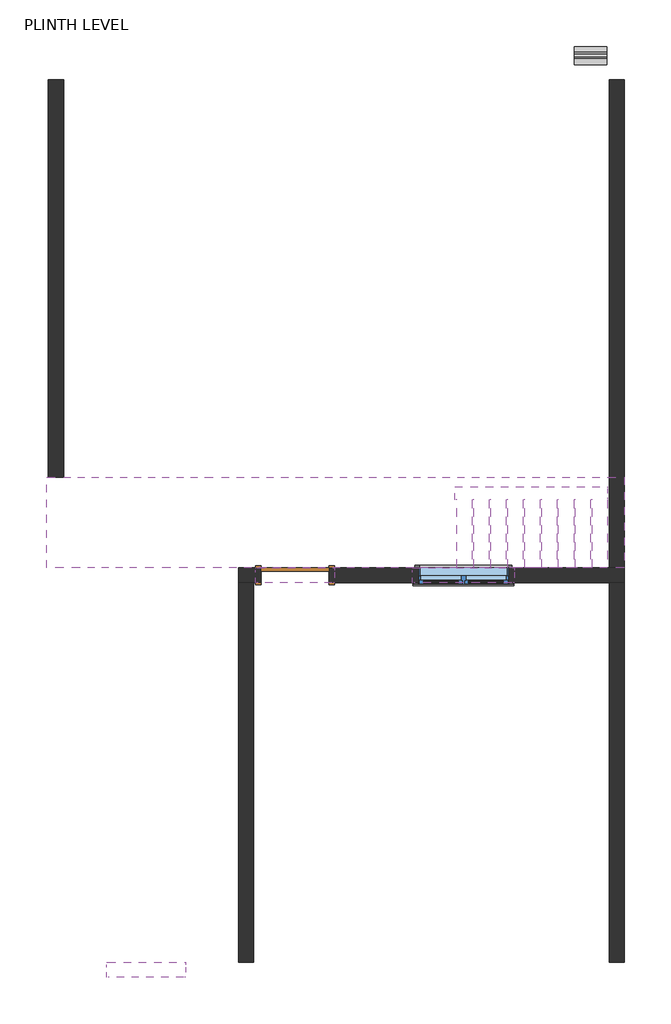
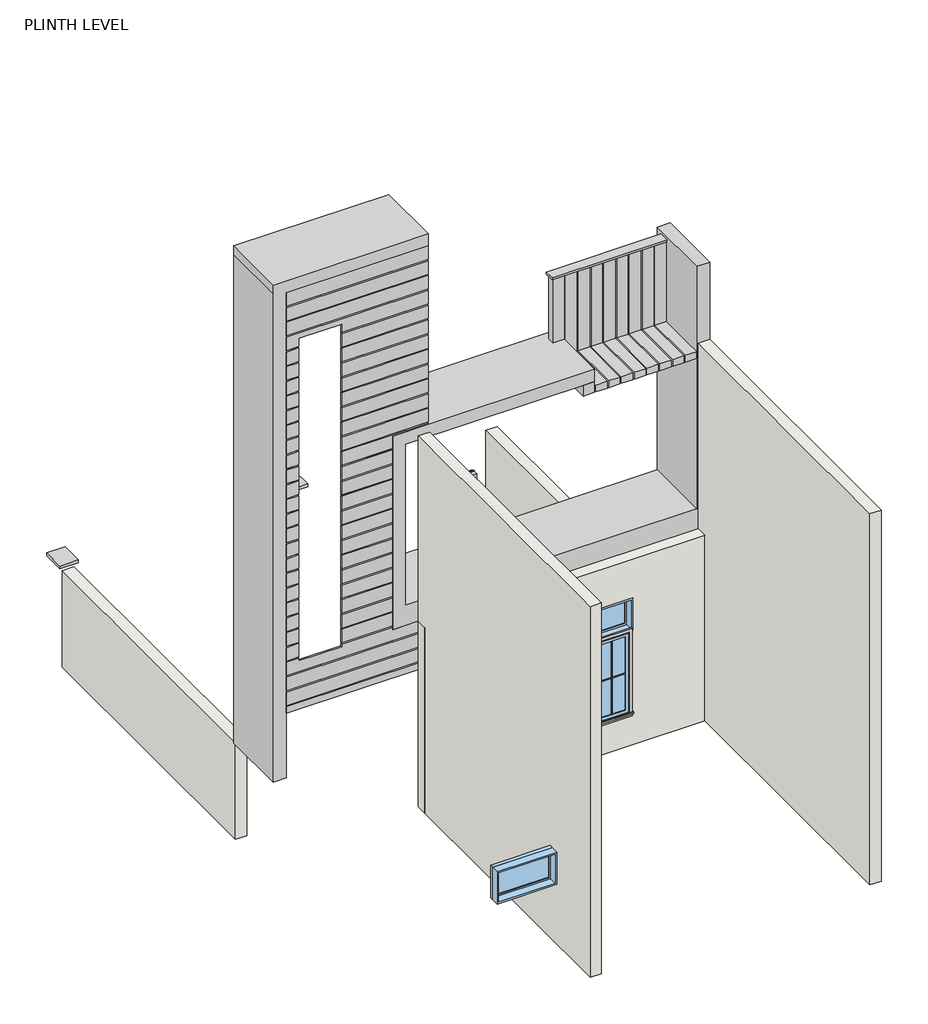
# One storey: 6 proxies, 5 walls, 4 windows, 1 door, 1 light fixture.
"""IFC4 building model written with IfcOpenShell, lengths in millimetres."""

from ifc_helpers import new_model, si_unit, frame, origin, place, context, project, spatial, polyline, outline, extrude, faceted_brep, transform, mapped, element, save
from components import generic_models_4_generic_models_4_1a732ec2, generic_models_6_generic_models_6_807765a8, muntin_pattern_2x2_muntin_pattern_2x2_6dad3731, muntin_pattern_2x2_muntin_pattern_2x2_a30a3345, trim_window_exterior_flat_with_sill_e3be2e48, trim_window_interior_flat_picture_frame_1906adc9, door_54dd4da4, wall_pack_light_exterior_120v_663ef98a, window_e8893895, window_5b0cf282, window_f2c349b1

model = new_model("IFC4")

# Units and contexts
model_context = context("Model", 3, world=origin())
ifc_project = project(units=[si_unit("LENGTHUNIT", "METRE", prefix="MILLI")], contexts=[model_context])

# Site, building, storey
site = spatial("IfcSite", under=ifc_project)
building = spatial("IfcBuilding", under=site)
storey = spatial("IfcBuildingStorey", under=building, Name="PLINTH LEVEL", Elevation=914.4)

# Proxies
placement = place(None, origin())
generic_models_4_generic_models_4_shape = generic_models_4_generic_models_4_1a732ec2(model_context)
element("IfcBuildingElementProxy", 1, Name="Generic Models 4 : Generic Models 4", ObjectType="Generic Models 4 : Generic Models 4", at=placement, inside=storey, context=model_context, shape_type="MappedRepresentation", body=[
    mapped(generic_models_4_generic_models_4_shape, transform((0.0, 0.0, 0.0), x_axis=(1.0, 0.0, 0.0), y_axis=(0.0, 1.0, 0.0), z_axis=(0.0, 0.0, 1.0))),
])
generic_models_6_generic_models_6_shape = generic_models_6_generic_models_6_807765a8(model_context)
element("IfcBuildingElementProxy", 2, Name="Generic Models 6 : Generic Models 6", ObjectType="Generic Models 6 : Generic Models 6", at=placement, inside=storey, context=model_context, shape_type="MappedRepresentation", body=[
    mapped(generic_models_6_generic_models_6_shape, transform((0.0, 0.0, 0.0), x_axis=(1.0, 0.0, 0.0), y_axis=(0.0, 1.0, 0.0), z_axis=(0.0, 0.0, 1.0))),
])
muntin_pattern_2x2_muntin_pattern_2x2_shape = muntin_pattern_2x2_muntin_pattern_2x2_6dad3731(model_context)
element("IfcBuildingElementProxy", 3, Name="Muntin Pattern_2x2 : Muntin Pattern_2x2", ObjectType="Muntin Pattern_2x2 : Muntin Pattern_2x2", at=placement, inside=storey, context=model_context, shape_type="MappedRepresentation", body=[
    mapped(muntin_pattern_2x2_muntin_pattern_2x2_shape, transform((-13781.656205, -12333.7777976, 1619.25), x_axis=(-1.0, 0.0, 0.0), y_axis=(0.0, -1.0, 0.0), z_axis=(0.0, 0.0, 1.0))),
])
muntin_pattern_2x2_muntin_pattern_2x2_2_shape = muntin_pattern_2x2_muntin_pattern_2x2_a30a3345(model_context)
element("IfcBuildingElementProxy", 4, Name="Muntin Pattern_2x2 : Muntin Pattern_2x2", ObjectType="Muntin Pattern_2x2 : Muntin Pattern_2x2", at=placement, inside=storey, context=model_context, shape_type="MappedRepresentation", body=[
    mapped(muntin_pattern_2x2_muntin_pattern_2x2_2_shape, transform((-14388.081205, -12333.7777976, 1619.25), x_axis=(1.0, 0.0, 0.0), y_axis=(0.0, 1.0, 0.0), z_axis=(0.0, 0.0, 1.0))),
])
trim_window_exterior_flat_with_sill_shape = trim_window_exterior_flat_with_sill_e3be2e48(model_context)
element("IfcBuildingElementProxy", 5, Name="Trim-Window-Exterior-Flat : with Sill", ObjectType="Trim-Window-Exterior-Flat : with Sill", at=placement, inside=storey, context=model_context, shape_type="MappedRepresentation", body=[
    mapped(trim_window_exterior_flat_with_sill_shape, transform((-14084.868705, -12343.3027976, 3073.4), x_axis=(-1.0, 0.0, 0.0), y_axis=(0.0, 0.0, -1.0), z_axis=(0.0, -1.0, 0.0))),
])
trim_window_interior_flat_picture_frame_shape = trim_window_interior_flat_picture_frame_1906adc9(model_context)
element("IfcBuildingElementProxy", 6, Name="Trim-Window-Interior-Flat : Picture Frame", ObjectType="Trim-Window-Interior-Flat : Picture Frame", at=placement, inside=storey, context=model_context, shape_type="MappedRepresentation", body=[
    mapped(trim_window_interior_flat_picture_frame_shape, transform((-14084.868705, -12140.1027976, 3073.4), x_axis=(1.0, 0.0, 0.0), y_axis=(0.0, 0.0, -1.0), z_axis=(0.0, 1.0, 0.0))),
])

# Door
door_shape = door_54dd4da4(model_context)
element("IfcDoor", 7, ObjectType="Single-Flush : 36\" x 84\"", at=placement, inside=storey, context=model_context, shape_type="MappedRepresentation", body=[
    mapped(door_shape, transform((-16358.168705, -12241.7027976, 914.4), x_axis=(1.0, 0.0, 0.0), y_axis=(0.0, 1.0, 0.0), z_axis=(0.0, 0.0, 1.0))),
])

# Light fixture
wall_pack_light_exterior_120v_shape = wall_pack_light_exterior_120v_663ef98a(model_context)
element("IfcLightFixture", 8, ObjectType="Wall Pack Light - Exterior : 120V", at=placement, inside=storey, context=model_context, shape_type="MappedRepresentation", body=[
    mapped(wall_pack_light_exterior_120v_shape, transform((-12492.1327615, -5459.9027976, -1390.9222814), x_axis=(1.0, 0.0, 0.0), y_axis=(0.0, 1.0, 0.0), z_axis=(0.0, 0.0, 1.0))),
])

# Walls
element("IfcWall", 9, ObjectType="Generic - 8\"", at=placement, inside=storey, context=model_context, shape_type="SweptSolid", body=[
    extrude(outline(polyline([(-12116.368705, -12140.1027976), (-12116.368705, -5561.5027976), (-11913.168705, -5561.5027976), (-11913.168705, -12140.1027976), (-12116.368705, -12140.1027976)])), frame((0.0, 0.0, 914.4), z_axis=(0.0, 0.0, 1.0), x_axis=(1.0, 0.0, 0.0)), (0.0, 0.0, 1.0), 1371.6),
])
element("IfcWall", 10, ObjectType="Generic - 8\"", at=placement, inside=storey, context=model_context, shape_type="SweptSolid", body=[
    extrude(outline(polyline([(-19482.368705, -5561.5027976), (-19482.368705, -10920.9027976), (-19685.568705, -10920.9027976), (-19685.568705, -5561.5027976), (-19482.368705, -5561.5027976)])), frame((0.0, 0.0, 457.2), z_axis=(0.0, 0.0, 1.0), x_axis=(1.0, 0.0, 0.0)), (0.0, 0.0, 1.0), 1828.8),
])
element("IfcWall", 11, ObjectType="Generic - 8\"", at=placement, inside=storey, context=model_context, shape_type="Brep", body=[
    faceted_brep([(-11913.168705, -17461.4027976, 914.4), (-11913.168705, -12343.3027976, 914.4), (-11913.168705, -12343.3027976, 4419.6), (-11913.168705, -12140.1027976, 4419.6), (-11913.168705, -12140.1027976, 7924.8), (-11913.168705, -17461.4027976, 7924.8), (-12116.368705, -17461.4027976, 914.4), (-12116.368705, -17461.4027976, 7924.8), (-12116.368705, -12343.3027976, 7924.8), (-12116.368705, -12140.1027976, 7924.8), (-12116.368705, -12140.1027976, 4419.6), (-12116.368705, -12343.3027976, 4419.6), (-12116.368705, -12343.3027976, 914.4)], [[[0, 1, 2, 3, 4, 5]], [[6, 7, 8, 9, 10, 11, 12]], [[1, 0, 6, 12]], [[5, 4, 9, 8, 7]], [[0, 5, 7, 6]], [[10, 3, 2, 11]], [[2, 1, 12, 11]], [[4, 3, 10, 9]]]),
])
element("IfcWall", 12, ObjectType="Generic - 8\"", at=placement, inside=storey, context=model_context, shape_type="Brep", body=[
    faceted_brep([(-17120.168705, -12343.3027976, 4419.6), (-17120.168705, -12343.3027976, 914.4), (-17120.168705, -17461.4027976, 914.4), (-17120.168705, -17461.4027976, 7924.8), (-17120.168705, -12140.1027976, 7924.8), (-17120.168705, -12140.1027976, 4419.6), (-16916.968705, -12343.3027976, 914.4), (-16916.968705, -12343.3027976, 4419.6), (-16916.968705, -12140.1027976, 4419.6), (-16916.968705, -12140.1027976, 7924.8), (-16916.968705, -12343.3027976, 7924.8), (-16916.968705, -17461.4027976, 7924.8), (-16916.968705, -17461.4027976, 914.4)], [[[0, 1, 2, 3, 4, 5]], [[6, 7, 8, 9, 10, 11, 12]], [[2, 1, 6, 12]], [[4, 3, 11, 10, 9]], [[5, 8, 7, 0]], [[0, 7, 6, 1]], [[5, 4, 9, 8]], [[3, 2, 12, 11]]]),
])
element("IfcWall", 13, ObjectType="Generic - 8\" 2", at=placement, inside=storey, context=model_context, shape_type="Brep", body=[
    faceted_brep([(-17120.168705, -12140.1027976, 4419.6), (-16916.968705, -12140.1027976, 4419.6), (-16815.368705, -12140.1027976, 4419.6), (-15900.968705, -12140.1027976, 4419.6), (-12116.368705, -12140.1027976, 4419.6), (-11913.168705, -12140.1027976, 4419.6), (-11913.168705, -12140.1027976, 2286.0), (-11913.168705, -12140.1027976, 914.4), (-12116.368705, -12140.1027976, 914.4), (-15900.968705, -12140.1027976, 914.4), (-15900.968705, -12140.1027976, 3048.0), (-16815.368705, -12140.1027976, 3048.0), (-16815.368705, -12140.1027976, 914.4), (-17120.168705, -12140.1027976, 914.4), (-17120.168705, -12140.1027976, 3505.2), (-15824.768705, -12140.1027976, 3067.05), (-15824.768705, -12140.1027976, 3676.65), (-16891.568705, -12140.1027976, 3676.65), (-16891.568705, -12140.1027976, 3067.05), (-13399.068705, -12140.1027976, 3073.4), (-13399.068705, -12140.1027976, 3683.0), (-14770.668705, -12140.1027976, 3683.0), (-14770.668705, -12140.1027976, 3073.4), (-14694.468705, -12140.1027976, 3073.4), (-14694.468705, -12140.1027976, 1549.4), (-13475.268705, -12140.1027976, 1549.4), (-13475.268705, -12140.1027976, 3073.4), (-11913.168705, -12343.3027976, 4419.6), (-12116.368705, -12343.3027976, 4419.6), (-15900.968705, -12343.3027976, 4419.6), (-16815.368705, -12343.3027976, 4419.6), (-16916.968705, -12343.3027976, 4419.6), (-17120.168705, -12343.3027976, 4419.6), (-17120.168705, -12343.3027976, 3505.2), (-17120.168705, -12343.3027976, 914.4), (-16916.968705, -12343.3027976, 914.4), (-16815.368705, -12343.3027976, 914.4), (-16815.368705, -12343.3027976, 3048.0), (-15900.968705, -12343.3027976, 3048.0), (-15900.968705, -12343.3027976, 914.4), (-12116.368705, -12343.3027976, 914.4), (-11913.168705, -12343.3027976, 914.4), (-15824.768705, -12343.3027976, 3676.65), (-15824.768705, -12343.3027976, 3067.05), (-16891.568705, -12343.3027976, 3067.05), (-16891.568705, -12343.3027976, 3676.65), (-13399.068705, -12343.3027976, 3683.0), (-13399.068705, -12343.3027976, 3073.4), (-13475.268705, -12343.3027976, 3073.4), (-13475.268705, -12343.3027976, 1549.4), (-14694.468705, -12343.3027976, 1549.4), (-14694.468705, -12343.3027976, 3073.4), (-14770.668705, -12343.3027976, 3073.4), (-14770.668705, -12343.3027976, 3683.0)], [[[0, 1, 2, 3, 4, 5, 6, 7, 8, 9, 10, 11, 12, 13, 14], [15, 16, 17, 18], [19, 20, 21, 22, 23, 24, 25, 26]], [[27, 28, 29, 30, 31, 32, 33, 34, 35, 36, 37, 38, 39, 40, 41], [42, 43, 44, 45], [46, 47, 48, 49, 50, 51, 52, 53]], [[39, 9, 8, 7, 41, 40]], [[12, 36, 35, 34, 13]], [[5, 4, 3, 2, 1, 0, 32, 31, 30, 29, 28, 27]], [[10, 9, 39, 38]], [[11, 10, 38, 37]], [[12, 11, 37, 36]], [[42, 16, 15, 43]], [[43, 15, 18, 44]], [[44, 18, 17, 45]], [[16, 42, 45, 17]], [[47, 46, 20, 19]], [[47, 19, 26, 48]], [[22, 52, 51, 23]], [[53, 52, 22, 21]], [[46, 53, 21, 20]], [[25, 49, 48, 26]], [[49, 25, 24, 50]], [[50, 24, 23, 51]], [[5, 27, 41, 7, 6]], [[13, 34, 33, 32, 0, 14]]]),
])

# Windows
window_shape = window_e8893895(model_context)
element("IfcWindow", 14, ObjectType="Fixed : 42\" x 24\"", at=placement, inside=storey, context=model_context, shape_type="MappedRepresentation", body=[
    mapped(window_shape, transform((-18326.668705, -17563.0027976, 914.4), x_axis=(1.0, 0.0, 0.0), y_axis=(0.0, 1.0, 0.0), z_axis=(0.0, 0.0, 1.0))),
])
element("IfcWindow", 15, ObjectType="Fixed : 42\" x 24\"", at=placement, inside=storey, context=model_context, shape_type="MappedRepresentation", body=[
    mapped(window_shape, transform((-16320.068705, -12241.7027976, 933.45), x_axis=(1.0, 0.0, 0.0), y_axis=(0.0, 1.0, 0.0), z_axis=(0.0, 0.0, 1.0))),
])
window_2_shape = window_5b0cf282(model_context)
element("IfcWindow", 16, ObjectType="Fixed : 54\" x 24\"", at=placement, inside=storey, context=model_context, shape_type="MappedRepresentation", body=[
    mapped(window_2_shape, transform((-14046.768705, -12241.7027976, 939.8), x_axis=(1.0, 0.0, 0.0), y_axis=(0.0, 1.0, 0.0), z_axis=(0.0, 0.0, 1.0))),
])
window_3_shape = window_f2c349b1(model_context)
element("IfcWindow", 17, ObjectType="Window-Casement-Double : 48\" x 60\"", at=placement, inside=storey, context=model_context, shape_type="MappedRepresentation", body=[
    mapped(window_3_shape, transform((-14084.868705, -12241.7027976, 635.0), x_axis=(1.0, 0.0, 0.0), y_axis=(0.0, 1.0, 0.0), z_axis=(0.0, 0.0, 1.0))),
])

save(model, "model.ifc")

# Revit data of these elements
# Type "Muntin Pattern_2x2 : Muntin Pattern_2x2"
#   Width [instance default] = 4' - 0"
#   Thickness = 0' - 0 1/2"
#   Height [instance default] = 4' - 0"
#   Distance = 0' - 0 3/4"
#   Interior Material [instance default] = none
#   Exterior Material [instance default] = none
#   Default Elevation = 0
# Type "Trim-Window-Exterior-Flat : with Sill"
#   Trim Width = 0' - 2 1/4"
#   Trim Thickness_Picture Frame = 0' - 1 1/4"
#   Trim Thickness_with Sill = 0' - 0 3/4"
#   Sill Thickness = 0' - 1 1/4"
#   Opening Width [instance default] = 2' - 0"
#   Opening Height [instance default] = 3' - 0"
#   Default Elevation = 4' - 0"
#   Sill = yes
#   Picture Frame = no
#   Trim Material [instance default] = none
# Type "Trim-Window-Interior-Flat : Picture Frame"
#   Trim Thickness_Picture Frame = 0' - 1 1/4"
#   Trim Width = 0' - 2 1/4"
#   Trim Thickness_with Sill = 0' - 0 3/4"
#   Sill Thickness = 0' - 1 1/4"
#   Opening Width [instance default] = 2' - 0"
#   Opening Height [instance default] = 3' - 0"
#   Default Elevation = 4' - 0"
#   Sill = no
#   Picture Frame = yes
#   Trim Material [instance default] = none
# Type "Single-Flush : 36\" x 84\""
#   Type Mark = "1"
#   Construction Type Id = "MDOOR"
#   Assembly Code = "C1020"
#   Analytic Construction = "Metal"
#   Thickness = 0' - 2"
#   Heat Transfer Coefficient (U) = 0.651978 BTU/(h·ft²·°F)
#   Height = 7' - 0"
#   Trim Projection Ext = 0' - 1"
#   Trim Projection Int = 0' - 1"
#   Trim Width = 0' - 3"
#   Width = 3' - 0"
#   Define Thermal Properties by = 1
#   Define Thermal Properties by = 1
#   Door Material = Door - Panel
#   Frame Material = Door - Frame
#   Visual Light Transmittance = 0
#   Solar Heat Gain Coefficient = 0
#   Function = (empty or 0)
#   Wall Closure = (empty or 0)
# Type "Wall Pack Light - Exterior : 120V"
#   Assembly Code = "D5020230"
#   Wattage = 300 W
#   built-in parameter 1150110 = 1 (stored number, unit not read)
#   built-in parameter 1114217 = 1 (stored number, unit not read)
#   built-in parameter 1150109 = 1 (stored number, unit not read)
#   built-in parameter 1150113 = 1 (stored number, unit not read)
#   built-in parameter 1150115 = 1 (stored number, unit not read)
#   built-in parameter 1150105 = 1875.72 (stored number, unit not read)
#   Light Source Symbol Size = 2' - 0"
#   built-in parameter 1150112 = 1 (stored number, unit not read)
#   built-in parameter 1150114 = 1 (stored number, unit not read)
#   built-in parameter 1150107 = 4000 (stored number, unit not read)
#   built-in parameter 1150106 = 18.7572 (stored number, unit not read)
#   built-in parameter 1150104 = 7.29939 (stored number, unit not read)
#   Ballast Voltage = 120 V
#   built-in parameter 1114218 = 1 (stored number, unit not read)
#   built-in parameter 1150133 = 10 (stored number, unit not read)
#   Lumens = 23571 lm
#   Mounting Height = 9' - 0"
#   Apparent Load = 70 VA
#   built-in parameter 1150134 = 12
#   built-in parameter 1150137 = 1
#   Color Filter = 16777215
#   Ballast Number of Poles = 1
#   Wall Mount Material = Metal - Paint Finish - Dark Grey, Matte
#   Shade Material = Glass
#   Load Classification = Lighting - Exterior
#   Dimming Lamp Color Temperature Shift = (empty or 0)
#   Default Elevation = 0
# Type "Generic - 8\""
#   Assembly Code = "B2010"
#   Layers, outside or top first: 0' - 8" no material (function 1)
# Type "Generic - 8\" 2"
#   Assembly Code = "B2010"
# Type "Fixed : 42\" x 24\""
#   Type Mark = "18"
#   Construction Type Id = "GSP4R"
#   Assembly Code = "B2020100"
#   Analytic Construction = "1/8 in Pilkington single glazing"
#   Visual Light Transmittance = 0.9
#   Solar Heat Gain Coefficient = 0.78
#   Heat Transfer Coefficient (U) = 0.6496 BTU/(h·ft²·°F)
#   Height = 2' - 0"
#   Default Sill Height = 7' - 0"
#   Width = 3' - 6"
#   Window Inset = 0' - 0 3/4"
#   Define Thermal Properties by = 1
#   Glass Pane Material = Glass
#   Sash Material = Sash
#   Wall Closure = (empty or 0)
# Type "Fixed : 54\" x 24\""
#   Type Mark = "20"
#   Construction Type Id = "GSP4R"
#   Assembly Code = "B2020100"
#   Analytic Construction = "1/8 in Pilkington single glazing"
#   Visual Light Transmittance = 0.9
#   Solar Heat Gain Coefficient = 0.78
#   Heat Transfer Coefficient (U) = 0.6496 BTU/(h·ft²·°F)
#   Height = 2' - 0"
#   Default Sill Height = 7' - 0"
#   Width = 4' - 6"
#   Window Inset = 0' - 0 3/4"
#   Define Thermal Properties by = 1
#   Glass Pane Material = Glass
#   Sash Material = Sash
#   Wall Closure = (empty or 0)
# Type "Window-Casement-Double : 48\" x 60\""
#   Type Mark = "16"
#   Fire Rating = "0.5h"
#   Assembly Code = "B2020100"
#   Analytic Construction = "Double glazing - domestic"
#   Frame Extension [instance default] = 0' - 0 1/4"
#   Window Inset [instance default] = 0' - 0"
#   Wall Thickness [instance default] = 0' - 6"
#   Interior Wall Closure [instance default] = 0' - 2 1/4"
#   Half Width = 2' - 0"
#   Visual Light Transmittance = 0.81
#   Thermal Resistance (R) = 1.8146 (h·ft²·°F)/BTU
#   Solar Heat Gain Coefficient = 0.76
#   Rough Width = 4' - 0 1/2"
#   Rough Height = 5' - 0 1/2"
#   Height = 5' - 0"
#   Heat Transfer Coefficient (U) = 0.5511 BTU/(h·ft²·°F)
#   Exterior Wall Closure [instance default] = 0' - 1 1/4"
#   Extension Jamb [instance default] = 0' - 2 1/4"
#   Default Sill Height = 3' - 0"
#   Width = 4' - 0"
#   Define Thermal Properties by = 0
#   Muntin Visibility = yes
#   Interior Trim Visibility [instance default] = yes
#   Exterior Trim Visibility [instance default] = yes
#   Extension Jamb Visibility [instance default] = yes
#   Interior Trim Material = Wood - Stained
#   Muntin Pattern = Muntin Pattern_2x2 : Muntin Pattern_2x2
#   Interior Trim = Trim-Window-Interior-Flat : Picture Frame
#   Interior Frame Material = Wood - Stained
#   Glass Panel Material = Glass
#   Exterior Trim Material = Clad - White
#   Exterior Trim = Trim-Window-Exterior-Flat : with Sill
#   Exterior Frame Material = Clad - White
#   Wall Closure = (empty or 0)
# Element 1 (IfcBuildingElementProxy, "Generic Models 4 : Generic Models 4")
#   Phase Created = New Construction
#   Materials on its faces: "Softwood, Lumber", "Gypsum Wall Board"
# Element 2 (IfcBuildingElementProxy, "Generic Models 6 : Generic Models 6")
#   Phase Created = New Construction
#   Materials on its faces: "Wood Planks"
# Elements 3, 4 (IfcBuildingElementProxy, "Muntin Pattern_2x2 : Muntin Pattern_2x2")
#   Width = 1' - 6 5/8"
#   Height = 4' - 6 1/2"
#   Interior Material = Wood - Stained
#   Exterior Material = Clad - White
#   Phase Created = New Construction
#   Materials on its faces: "Clad - White", "Wood - Stained"
# Element 5 (IfcBuildingElementProxy, "Trim-Window-Exterior-Flat : with Sill")
#   Opening Width = 4' - 0"
#   Opening Height = 5' - 0"
#   Trim Material = Clad - White
#   Phase Created = New Construction
#   Materials on its faces: "Clad - White"
# Element 6 (IfcBuildingElementProxy, "Trim-Window-Interior-Flat : Picture Frame")
#   Opening Width = 4' - 0"
#   Opening Height = 5' - 0"
#   Trim Material = Wood - Stained
#   Phase Created = New Construction
#   Materials on its faces: "Wood - Stained"
# Element 7 (IfcDoor, "Single-Flush : 36\" x 84\"")
#   Phase Created = New Construction
#   Materials on its faces: "Door - Frame", "Door - Panel"
# Element 8 (IfcLightFixture, "Wall Pack Light - Exterior : 120V")
#   Mark = "1"
#   Phase Created = New Construction
#   Materials on its faces: "Metal - Paint Finish - Dark Grey, Matte", "Glass"
# Element 9 (IfcWall, "Generic - 8\"")
#   Top Offset = 0' - 0"
#   Base Offset = 0' - 0"
#   Unconnected Height = 4' - 6"
#   wall height = 4' - 6"
#   Phase Created = New Construction
#   Base Constraint = PLINTH LEVEL
#   Materials on its faces: "Default Wall"
# Element 10 (IfcWall, "Generic - 8\"")
#   built-in parameter 1001111 = -1' - 6"
#   Top Offset = 0' - 0"
#   Base Offset = -1' - 6"
#   Unconnected Height = 6' - 0"
#   wall height = 6' - 0"
#   Phase Created = New Construction
#   Base Constraint = PLINTH LEVEL
#   Materials on its faces: "Default Wall"
# Elements 11, 12 (IfcWall, "Generic - 8\"")
#   Top Offset = 0' - 0"
#   Base Offset = 0' - 0"
#   wall height = 23' - 0"
#   Phase Created = New Construction
#   Base Constraint = PLINTH LEVEL
#   Top Constraint = ROOF LEVEL
#   Materials on its faces: "Default Wall"
# Element 13 (IfcWall, "Generic - 8\" 2")
#   Top Offset = 0' - 0"
#   Base Offset = 0' - 0"
#   wall height = 11' - 6"
#   Phase Created = New Construction
#   Base Constraint = PLINTH LEVEL
#   Top Constraint = FIRST FLOOR LEVEL
#   Materials on its faces: "Default Wall"
# Element 14 (IfcWindow, "Fixed : 42\" x 24\"")
#   Mark = "11"
#   Phase Created = New Construction
#   Materials on its faces: "Sash", "Glass"
# Element 15 (IfcWindow, "Fixed : 42\" x 24\"")
#   Mark = "1"
#   Phase Created = New Construction
#   Materials on its faces: "Sash", "Glass"
# Element 16 (IfcWindow, "Fixed : 54\" x 24\"")
#   Mark = "2"
#   Phase Created = New Construction
#   Materials on its faces: "Sash", "Glass"
# Element 17 (IfcWindow, "Window-Casement-Double : 48\" x 60\"")
#   Mark = "3"
#   Window Inset = 0' - 0"
#   Interior Wall Closure = 0' - 2 1/4"
#   Frame Extension = 0' - 0 1/4"
#   Exterior Wall Closure = 0' - 1 1/4"
#   Interior Trim Visibility = yes
#   Exterior Trim Visibility = yes
#   Phase Created = New Construction
#   Materials on its faces: "Wood - Stained", "Glass", "Clad - White"
# Materials
#   "Door - Panel": class "Wood", colour RGB 210 159 95, transparency 0, Cost = 0
#   "Door - Frame": colour RGB 118 70 51, transparency 0, Cost = 0
#   "Metal - Paint Finish - Dark Grey, Matte": class "Paint", colour RGB 98 98 98, transparency 0
#   "Glass": class "Glass", colour RGB 0 128 192, transparency 0.75, Description = "Soda Lime Glass", Cost = 0
#   "Sash": class "Wood", colour RGB 224 178 126, transparency 0, Cost = 0
#   "Wood - Stained": class "Wood", colour RGB 224 178 126, transparency 0, Cost = 0
#   "Clad - White": class "Wood", colour RGB 242 242 238, transparency 0, Cost = 0
#   "Softwood, Lumber": class "Wood", colour RGB 223 192 134, transparency 0, Description = "Pinus Echinata", Cost = 0
#   "Gypsum Wall Board": class "Generic", colour RGB 228 228 228, transparency 0, Description = "Gypsum Wall Board", Cost = 0
#   "Wood Planks": class "Wood", colour RGB 129 72 39, transparency 0, Description = "Physical material.", Cost = 0
#   "Default Wall": colour RGB 128 128 128, transparency 0, Cost = 0
